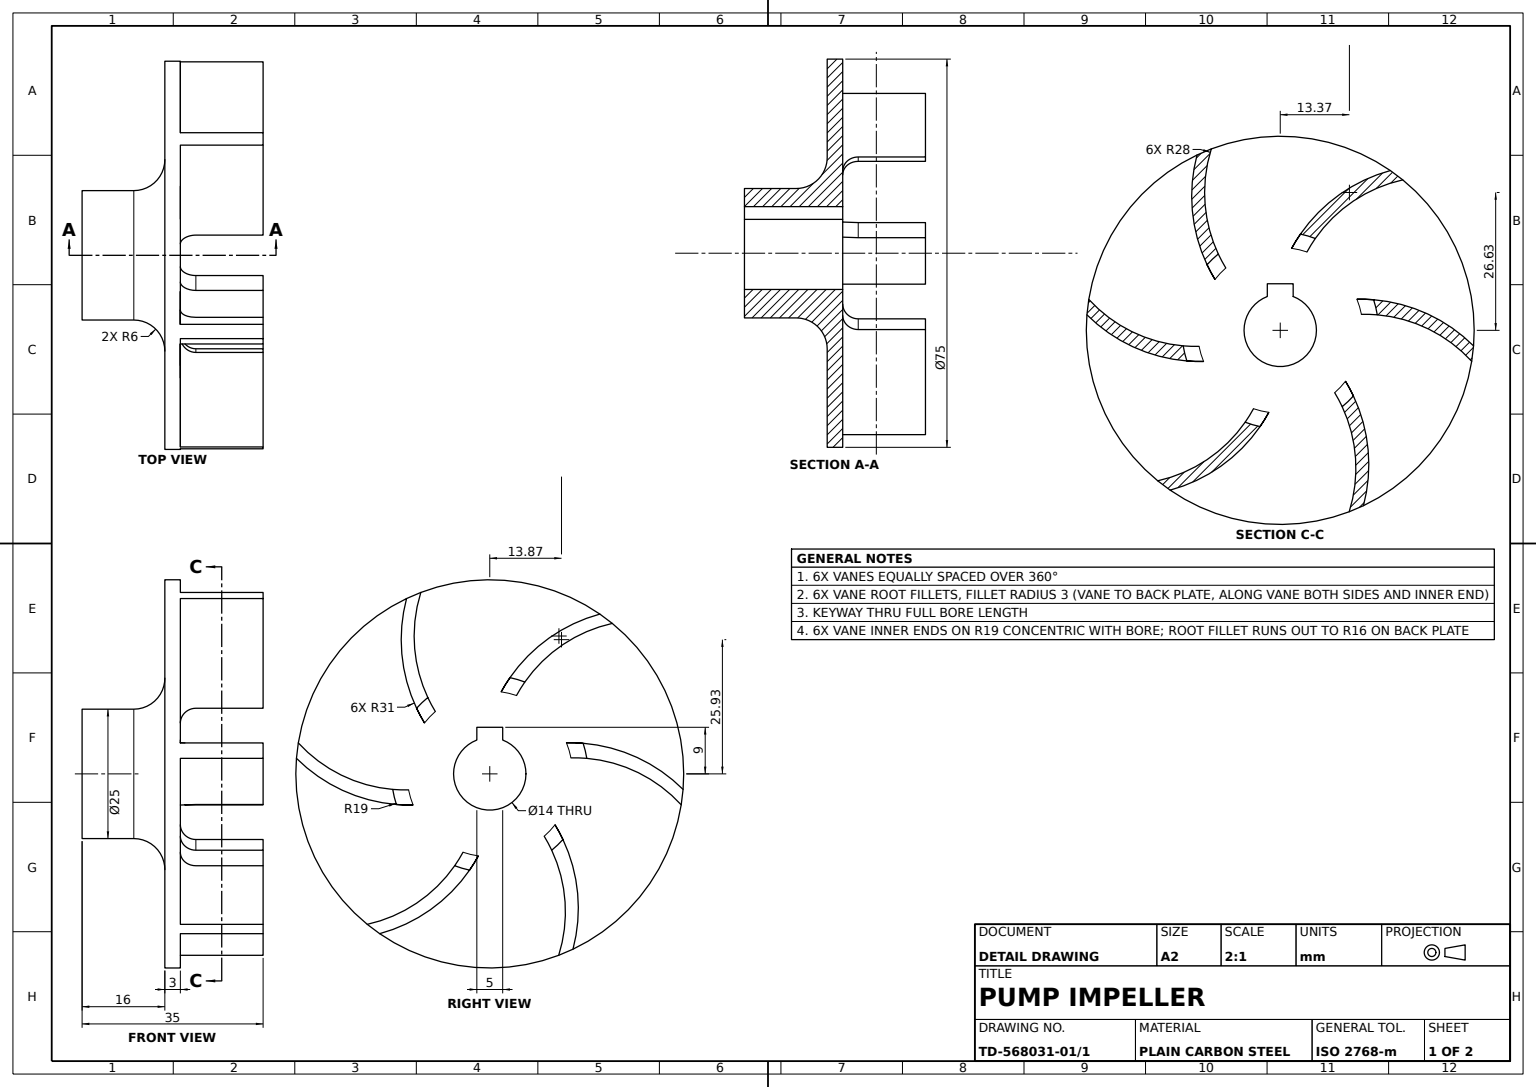
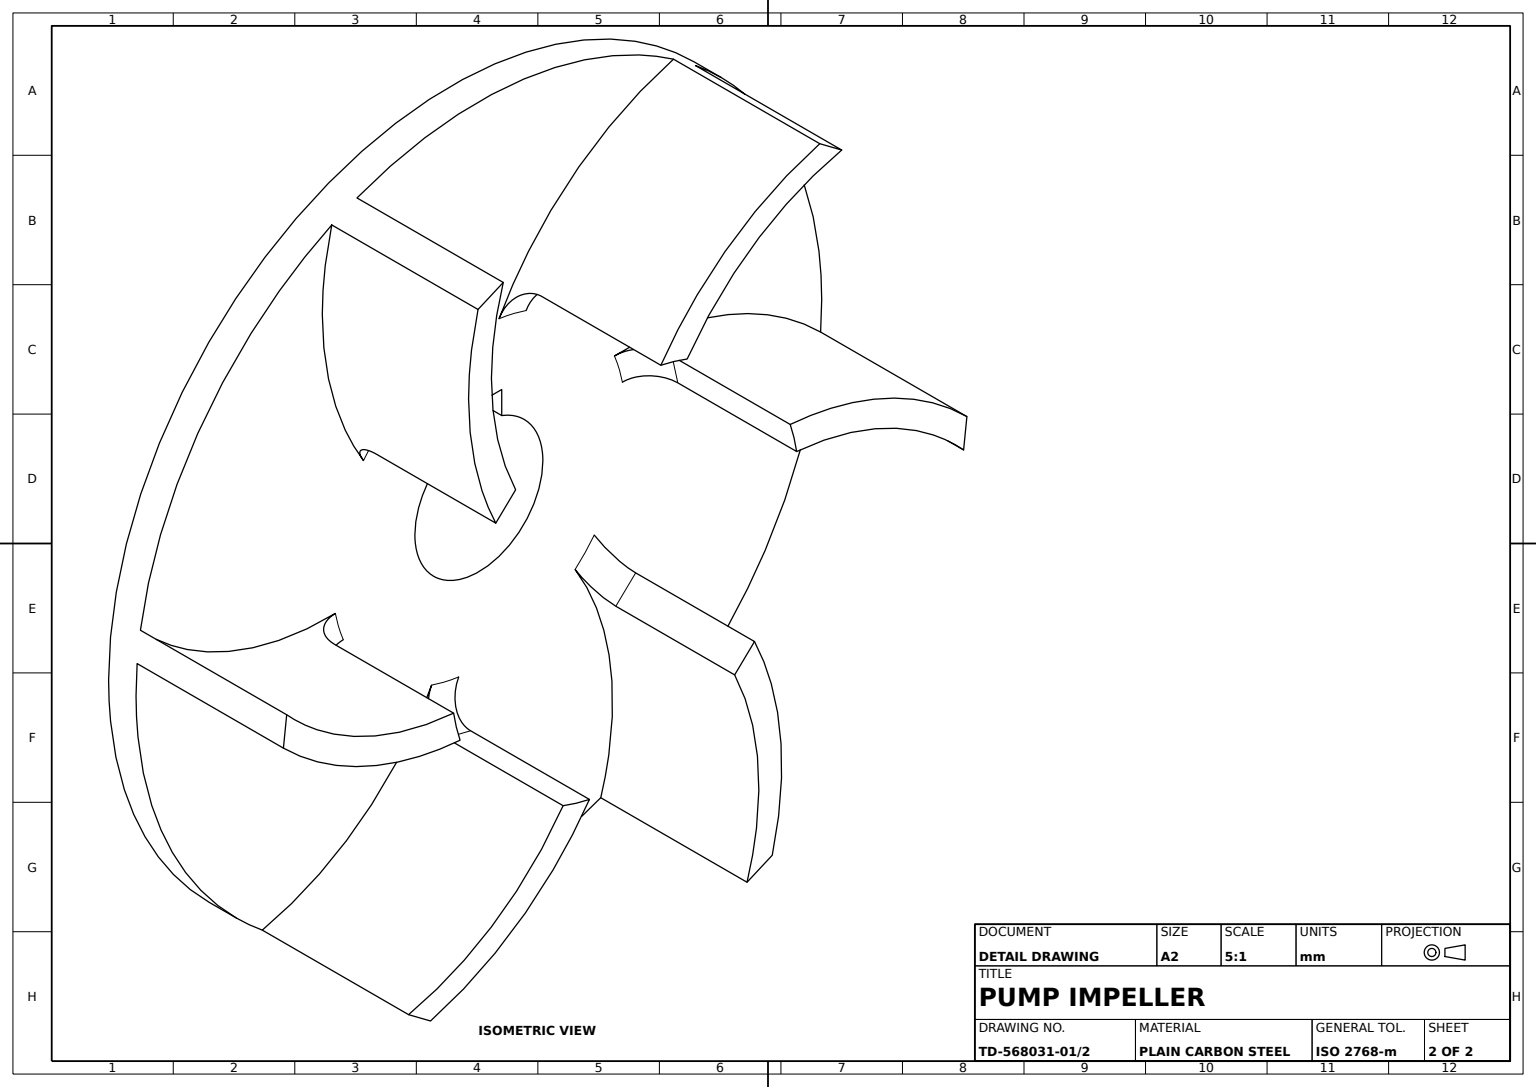
SolidWorks part; units mm, degrees
material "Plain Carbon Steel"
ref_plane "Front Plane" through (0, 0, 0) normal (0, 0, 1) x (1, 0, 0)
ref_plane "Top Plane" through (0, 0, 0) normal (0, 1, 0) x (1, 0, 0)
ref_plane "Right Plane" through (0, 0, 0) normal (1, 0, 0) x (0, 0, -1)
sketch "Back Plate Profile Sketch" plane through (0, 0, 0) normal (0, 0, 1) x (1, 0, 0)
  line L0 (0, 759.8465) -> (0, -759.8465) construction
  line L1 (-1406.5133, 0) -> (1010.027, 0) construction
  line L2 (-2.5, 9) -> (2.5, 9)
  line L3 (-2.5, 9) -> (-2.5, 6.5383)
  line L4 (2.5, 9) -> (2.5, 6.5383)
  circle A0 centre (0, 0) radius 37.5
  arc A1 (-2.5, 6.5383) -> (2.5, 6.5383) centre (0, 0) ccw
  dimension "D1" = 75
  dimension "D2" = 14
  dimension "D3" = 5
  dimension "D4" = 9
extrude "Back Plate Ø75" add sketch "Back Plate Profile Sketch" along normal mid plane 3 contours A0 A1 L3 L2 L4
sketch "Hub Sketch Ø25" plane through (0, 0, 1.5) normal (0, 0, 1) x (1, 0, 0)
  line L0 (-2.5, 9) -> (-2.5, 6.5383) construction
  line L1 (-2.5, 9) -> (2.5, 9) construction
  line L2 (2.5, 9) -> (2.5, 6.5383) construction
  line L3 (-2.5, 9) -> (-2.5, 6.5383)
  line L4 (-2.5, 9) -> (2.5, 9)
  line L5 (2.5, 9) -> (2.5, 6.5383)
  circle A0 centre (0, 0) radius 12.5
  arc A1 (-2.5, 6.5383) -> (2.5, 6.5383) centre (0, 0) ccw construction
  arc A2 (-2.5, 6.5383) -> (2.5, 6.5383) centre (0, 0) ccw
  arc M6 (2.5, 6.5383) -> (-2.5, 6.5383) centre (0, 0) cw
  line M7 (-2.5, 6.5383) -> (-2.5, 9)
  line M8 (-2.5, 9) -> (2.5, 9)
  line M9 (2.5, 9) -> (2.5, 6.5383)
  dimension "D1" = 25
extrude "Hub Ø25" add sketch "Hub Sketch Ø25" along normal blind 16 contours A0 M9 M6 M7 M8
fillet "Hub Root Fillet R6" radius 6 1 edges at (12.5, 0, 1.5)
sketch "Vane Profile Sketch" plane through (0, 0, -1.5) normal (0, 0, -1) x (-1, 0, 0)
  line L0 (-51.1116, 0) -> (55.2478, 0) construction
  line L1 (0, 44.7773) -> (0, -45.8409) construction
  line L2 (-52.6728, 3) -> (-14.3255, 3) construction
  line L3 (-52.6728, -3) -> (-14.3255, -3) construction
  line L4 (-2.5, 9) -> (-2.5, 6.5383) construction
  line L5 (2.5, 9) -> (-2.5, 9) construction
  arc A4 (-37.0204, 5.9784) -> (-18.7617, -3) centre (-16.3799, 24.8985) ccw
  arc A5 (-37.3798, 3) -> (-18.0556, -5.9157) centre (-15.5197, 24.9804) ccw
  arc A6 (-18.7617, -3) -> (-18.0556, -5.9157) centre (0, 0) ccw
  arc A7 (-37.0204, 5.9784) -> (-37.3798, 3) centre (0, 0) ccw
  point P14 (-18.7617, -3)
  point P15 (-18.0556, -5.9157)
  point P16 (-37.0204, 5.9784)
  point P17 (-37.3798, 3)
  dimension "D2" = 19
  dimension "D3" = 3
  dimension "D6" = 62
  dimension "D5" = 56
  dimension "D9" = 37.5
  dimension "D10" = 5.9784
  dimension "D13" = 2.5
  dimension "D1" = 3
  dimension "D4" = 3
  dimension "D7" = 24.9804
  dimension "D8" = 3
  dimension "D11" = 37.0204
  dimension "D12" = 37.3798
  dimension "D14" = 5
extrude "Vane" add sketch "Vane Profile Sketch" along normal blind 16
fillet "Vane Root Fillet R3" radius 3 1 edges at (18.4663, -4.4718, -1.5)
pattern_circular "Vane Pattern 6x" count 6 over 360 about axis through (0, 0, 0) along (0, 0, 1) of "Vane", "Vane Root Fillet R3"
